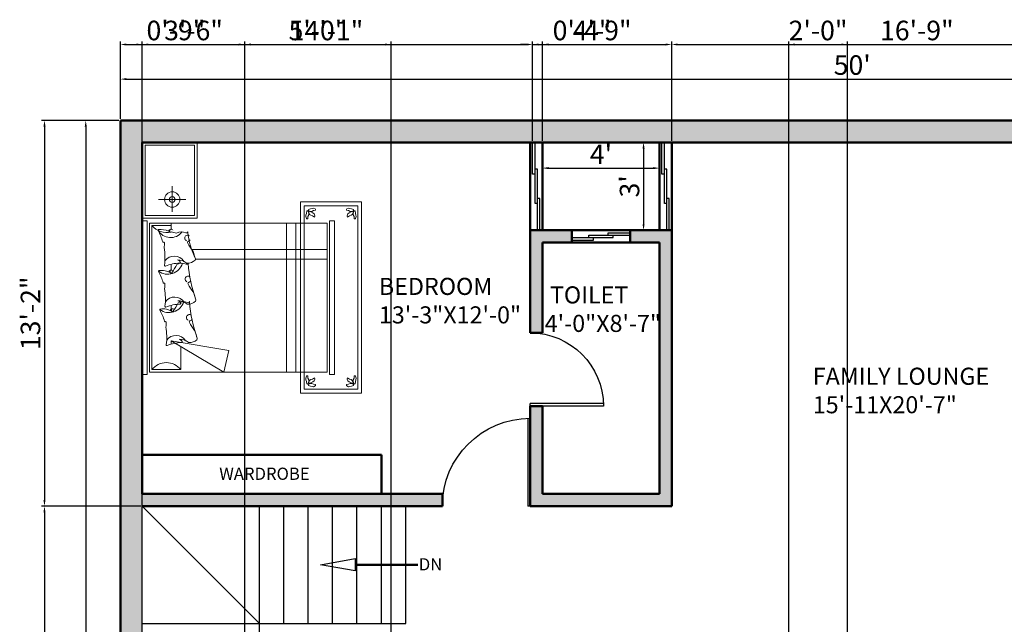
# Model space of a CAD drawing. Units: inches. Extents: x 1770 to 3141, y 984 to 1614.
# Tile 11 of 12: x 2468 to 2871, y 1359 to 1606. Entities that reach past the tile are written whole.
import ezdxf

# ---------------------------------------------------------------- set-up
doc = ezdxf.new("R2010")
doc.units = ezdxf.units.IN
for name, color, linetype, lineweight in [('A-ANNO-DIMS', 2, 'Continuous', 18), ('A-ANNO-TEXT', 7, 'Continuous', 18), ('A-AREA-IDEN', 3, 'Continuous', 18), ('A-DOOR', 4, 'Continuous', 25), ('A-FLOR-STRS', 7, 'Continuous', 25), ('A-FURN', 8, 'Continuous', 18), ('A-GLAZ', 5, 'Continuous', 25), ('A-WALL', 7, 'Continuous', 50), ('A-WALL-PATT', 8, 'Continuous', 13)]:
    doc.layers.add(name, color=color, linetype=linetype, lineweight=lineweight)
doc.styles.get("Standard").update_dxf_attribs({"font": 'arial.ttf'})
doc.dimstyles.new('ISO-25', dxfattribs={"dimtxt": 8, "dimasz": 2.5, "dimexe": 1.25, "dimexo": 0.625, "dimtad": 1, "dimdec": 1, "dimlunit": 3, "dimtxsty": 'Standard', "dimcen": 2.5, "dimclrt": 1, "dimadec": 0, "dimazin": 0, "dimtfac": 1, "dimtdec": 1, "dimtmove": 0, "dimatfit": 3, "dimfxl": 1, "dimarcsym": 0})

# ---------------------------------------------------------------- blocks, each defined once
blk = doc.blocks.new("D1 3'")
for p, q in [((0, 36), (0, 0)), ((1, 36), (1, 0)), ((0, 0), (1, 0))]:
    blk.add_line(p, q)
blk.add_arc((0, 0), 36, 0, 90)
blk = doc.blocks.new("D2 2'6")
for p, q in [((0, 30), (0, 0)), ((1, 30), (1, 0)), ((0, 0), (1, 0))]:
    blk.add_line(p, q)
blk.add_arc((0, 0), 30, 0, 90)
blk = doc.blocks.new('*D20')
at = {"layer": 'A-ANNO-DIMS', "color": 0, "lineweight": -2, "transparency": 16777216}
for p, q in [((2509.08, 1565.8), (2509.08, 1583.37)), ((3109.08, 1565.8), (3109.08, 1583.37)), ((2511.58, 1582.12), (3106.58, 1582.12))]:
    blk.add_line(p, q, dxfattribs=at)
at = {"layer": 'A-ANNO-DIMS', "color": 0, "transparency": 16777216}
for points in [[(2511.58, 1582.54), (2511.58, 1581.7), (2509.08, 1582.12)], [(3106.58, 1582.54), (3106.58, 1581.7), (3109.08, 1582.12)]]:
    blk.add_solid(points, dxfattribs=at)
at = {"layer": 'Defpoints', "color": 0, "transparency": 16777216}
for p in [(3109.08, 1582.12), (2509.08, 1565.18), (3109.08, 1565.18)]:
    blk.add_point(p, dxfattribs=at)
at = {"layer": 'A-ANNO-DIMS', "color": 0, "transparency": 16777216, "insert": (2809.08, 1586.83), "char_height": 8, "attachment_point": 5}
blk.add_mtext("50'", dxfattribs=at)
blk = doc.blocks.new('*D19')
at = {"layer": 'A-ANNO-DIMS', "color": 0, "lineweight": -2, "transparency": 16777216}
for p, q in [((2508.45, 1565.18), (2493.64, 1565.18)), ((2494.89, 1562.68), (2494.89, 1087.68)), ((2508.45, 1085.18), (2493.64, 1085.18))]:
    blk.add_line(p, q, dxfattribs=at)
at = {"layer": 'A-ANNO-DIMS', "color": 0, "transparency": 16777216}
for points in [[(2494.47, 1562.68), (2495.3, 1562.68), (2494.89, 1565.18)], [(2494.47, 1087.68), (2495.3, 1087.68), (2494.89, 1085.18)]]:
    blk.add_solid(points, dxfattribs=at)
at = {"layer": 'Defpoints', "color": 0, "transparency": 16777216}
for p in [(2509.08, 1565.18), (2494.89, 1085.18), (2509.08, 1085.18)]:
    blk.add_point(p, dxfattribs=at)
at = {"layer": 'A-ANNO-DIMS', "color": 0, "transparency": 16777216, "insert": (2490.18, 1325.18), "char_height": 8, "attachment_point": 5, "rotation": 90}
blk.add_mtext("40'", dxfattribs=at)
blk = doc.blocks.new('carpet-7')
at = {"color": 0, "linetype": 'ByBlock'}
for p, q in [((-1.0224, 0), (0, 0)), ((0, 0), (0, -0.54)), ((-1.694, -0.54), (-1.694, 0)), ((-1.694, 0), (-1.0224, 0)), ((-1.658, -0.5076), (-1.658, -0.0324)), ((-1.658, -0.0324), (-0.036, -0.0324)), ((-1.6304, -0.0896), (-1.6256, -0.0702)), ((-1.6256, -0.0702), (-1.6172, -0.0691)), ((-1.6172, -0.0691), (-1.6124, -0.0724)), ((-1.6112, -0.0562), (-1.6124, -0.0637)), ((-1.6124, -0.0637), (-1.6088, -0.068)), ((-1.6124, -0.0724), (-1.6064, -0.0886)), ((-1.5896, -0.0518), (-1.6112, -0.0562)), ((-1.6088, -0.068), (-1.5908, -0.0734)), ((-1.6088, -0.0788), (-1.6028, -0.0724)), ((-1.5992, -0.0961), (-1.6088, -0.0788)), ((-1.6028, -0.0724), (-1.5968, -0.0724)), ((-1.5968, -0.0724), (-1.5812, -0.081)), ((-1.5908, -0.0734), (-1.5764, -0.0724)), ((-1.5752, -0.0486), (-1.5896, -0.0518)), ((-1.5812, -0.081), (-1.5728, -0.0918)), ((-1.5764, -0.0724), (-1.5608, -0.0659)), ((-1.5608, -0.0464), (-1.5752, -0.0486)), ((-1.544, -0.0529), (-1.5608, -0.0464)), ((-1.5608, -0.0659), (-1.5404, -0.0637)), ((-1.5404, -0.0562), (-1.544, -0.0529)), ((-1.5404, -0.0637), (-1.5404, -0.0562)), ((-0.1512, -0.0562), (-0.1476, -0.0529)), ((-0.1512, -0.0637), (-0.1512, -0.0562)), ((-0.1308, -0.0659), (-0.1512, -0.0637)), ((-0.1476, -0.0529), (-0.1308, -0.0464)), ((-0.1308, -0.0464), (-0.1164, -0.0486)), ((-0.1152, -0.0724), (-0.1308, -0.0659)), ((-0.1104, -0.081), (-0.1188, -0.0918)), ((-0.1164, -0.0486), (-0.102, -0.0518)), ((-0.1008, -0.0734), (-0.1152, -0.0724)), ((-0.0948, -0.0724), (-0.1104, -0.081)), ((-0.102, -0.0518), (-0.0804, -0.0562)), ((-0.0828, -0.068), (-0.1008, -0.0734)), ((-0.0888, -0.0724), (-0.0948, -0.0724)), ((-0.0924, -0.0961), (-0.0828, -0.0788)), ((-0.0828, -0.0788), (-0.0888, -0.0724)), ((-0.0792, -0.0724), (-0.0852, -0.0886)), ((-0.0792, -0.0637), (-0.0828, -0.068)), ((-0.0804, -0.0562), (-0.0792, -0.0637)), ((-0.0744, -0.0691), (-0.0792, -0.0724)), ((-0.066, -0.0702), (-0.0744, -0.0691)), ((-0.0612, -0.0896), (-0.066, -0.0702)), ((-0.036, -0.0324), (-0.036, -0.5076)), ((-1.6364, -0.1156), (-1.634, -0.1026)), ((-1.6292, -0.1307), (-1.6364, -0.1156)), ((-1.634, -0.1026), (-1.6304, -0.0896)), ((-1.6256, -0.1339), (-1.6292, -0.1307)), ((-1.6172, -0.1339), (-1.6256, -0.1339)), ((-1.6148, -0.1156), (-1.6172, -0.1339)), ((-1.6076, -0.1015), (-1.6148, -0.1156)), ((-1.6064, -0.0886), (-1.6076, -0.1015)), ((-1.5932, -0.108), (-1.5992, -0.0961)), ((-1.5848, -0.1199), (-1.5932, -0.108)), ((-1.5692, -0.1274), (-1.5848, -0.1199)), ((-1.5728, -0.0918), (-1.568, -0.1069)), ((-1.5632, -0.1274), (-1.5692, -0.1274)), ((-1.568, -0.1069), (-1.5572, -0.1231)), ((-1.5572, -0.1231), (-1.5632, -0.1274)), ((-0.1236, -0.1069), (-0.1344, -0.1231)), ((-0.1344, -0.1231), (-0.1284, -0.1274)), ((-0.1284, -0.1274), (-0.1224, -0.1274)), ((-0.1188, -0.0918), (-0.1236, -0.1069)), ((-0.1224, -0.1274), (-0.1068, -0.1199)), ((-0.1068, -0.1199), (-0.0984, -0.108)), ((-0.0984, -0.108), (-0.0924, -0.0961)), ((-0.0852, -0.0886), (-0.084, -0.1015)), ((-0.084, -0.1015), (-0.0768, -0.1156)), ((-0.0768, -0.1156), (-0.0744, -0.1339)), ((-0.0744, -0.1339), (-0.066, -0.1339)), ((-0.066, -0.1339), (-0.0624, -0.1307)), ((-0.0624, -0.1307), (-0.0552, -0.1156)), ((-0.0576, -0.1026), (-0.0612, -0.0896)), ((-0.0552, -0.1156), (-0.0576, -0.1026)), ((-1.6292, -0.4093), (-1.6364, -0.4244)), ((-1.6364, -0.4244), (-1.634, -0.4374)), ((-1.6256, -0.4061), (-1.6292, -0.4093)), ((-1.6172, -0.4061), (-1.6256, -0.4061)), ((-1.6148, -0.4244), (-1.6172, -0.4061)), ((-1.6076, -0.4385), (-1.6148, -0.4244)), ((-1.5932, -0.432), (-1.5992, -0.4439)), ((-1.5848, -0.4201), (-1.5932, -0.432)), ((-1.5692, -0.4126), (-1.5848, -0.4201)), ((-1.5728, -0.4482), (-1.568, -0.4331)), ((-1.5632, -0.4126), (-1.5692, -0.4126)), ((-1.568, -0.4331), (-1.5572, -0.4169)), ((-1.5572, -0.4169), (-1.5632, -0.4126)), ((-0.1344, -0.4169), (-0.1284, -0.4126)), ((-0.1236, -0.4331), (-0.1344, -0.4169)), ((-0.1284, -0.4126), (-0.1224, -0.4126)), ((-0.1188, -0.4482), (-0.1236, -0.4331)), ((-0.1224, -0.4126), (-0.1068, -0.4201)), ((-0.1068, -0.4201), (-0.0984, -0.432)), ((-0.0984, -0.432), (-0.0924, -0.4439)), ((-0.084, -0.4385), (-0.0768, -0.4244)), ((-0.0768, -0.4244), (-0.0744, -0.4061)), ((-0.0744, -0.4061), (-0.066, -0.4061)), ((-0.066, -0.4061), (-0.0624, -0.4093)), ((-0.0624, -0.4093), (-0.0552, -0.4244)), ((-0.0552, -0.4244), (-0.0576, -0.4374)), ((-1.658, -0.5076), (-0.036, -0.5076)), ((-1.634, -0.4374), (-1.6304, -0.4504)), ((-1.6304, -0.4504), (-1.6256, -0.4698)), ((-1.6256, -0.4698), (-1.6172, -0.4709)), ((-1.6172, -0.4709), (-1.6124, -0.4676)), ((-1.6124, -0.4676), (-1.6064, -0.4514)), ((-1.6124, -0.4763), (-1.6088, -0.472)), ((-1.6112, -0.4838), (-1.6124, -0.4763)), ((-1.5896, -0.4882), (-1.6112, -0.4838)), ((-1.5992, -0.4439), (-1.6088, -0.4612)), ((-1.6088, -0.4612), (-1.6028, -0.4676)), ((-1.6088, -0.472), (-1.5908, -0.4666)), ((-1.6064, -0.4514), (-1.6076, -0.4385)), ((-1.6028, -0.4676), (-1.5968, -0.4676)), ((-1.5968, -0.4676), (-1.5812, -0.459)), ((-1.5908, -0.4666), (-1.5764, -0.4676)), ((-1.5752, -0.4914), (-1.5896, -0.4882)), ((-1.5812, -0.459), (-1.5728, -0.4482)), ((-1.5764, -0.4676), (-1.5608, -0.4741)), ((-1.5608, -0.4936), (-1.5752, -0.4914)), ((-1.5608, -0.4741), (-1.5404, -0.4763)), ((-1.544, -0.4871), (-1.5608, -0.4936)), ((-1.5404, -0.4838), (-1.544, -0.4871)), ((-1.5404, -0.4763), (-1.5404, -0.4838)), ((-0.1308, -0.4741), (-0.1512, -0.4763)), ((-0.1512, -0.4763), (-0.1512, -0.4838)), ((-0.1512, -0.4838), (-0.1476, -0.4871)), ((-0.1476, -0.4871), (-0.1308, -0.4936)), ((-0.1152, -0.4676), (-0.1308, -0.4741)), ((-0.1308, -0.4936), (-0.1164, -0.4914)), ((-0.1104, -0.459), (-0.1188, -0.4482)), ((-0.1164, -0.4914), (-0.102, -0.4882)), ((-0.1008, -0.4666), (-0.1152, -0.4676)), ((-0.0948, -0.4676), (-0.1104, -0.459)), ((-0.102, -0.4882), (-0.0804, -0.4838)), ((-0.0828, -0.472), (-0.1008, -0.4666)), ((-0.0888, -0.4676), (-0.0948, -0.4676)), ((-0.0924, -0.4439), (-0.0828, -0.4612)), ((-0.0828, -0.4612), (-0.0888, -0.4676)), ((-0.0852, -0.4514), (-0.084, -0.4385)), ((-0.0792, -0.4676), (-0.0852, -0.4514)), ((-0.0792, -0.4763), (-0.0828, -0.472)), ((-0.0804, -0.4838), (-0.0792, -0.4763)), ((-0.0744, -0.4709), (-0.0792, -0.4676)), ((-0.066, -0.4698), (-0.0744, -0.4709)), ((-0.0612, -0.4504), (-0.066, -0.4698)), ((-0.0576, -0.4374), (-0.0612, -0.4504)), ((0, -0.54), (-1.694, -0.54))]:
    blk.add_line(p, q, dxfattribs=at)
blk = doc.blocks.new('*D54')
at = {"layer": 'A-ANNO-DIMS', "color": 0, "lineweight": -2, "transparency": 16777216}
for p, q in [((2682.08, 1547.77), (2682.08, 1544.4)), ((2730.08, 1547.77), (2730.08, 1544.4)), ((2684.58, 1545.65), (2727.58, 1545.65))]:
    blk.add_line(p, q, dxfattribs=at)
at = {"layer": 'A-ANNO-DIMS', "color": 0, "transparency": 16777216}
for points in [[(2684.58, 1546.07), (2684.58, 1545.23), (2682.08, 1545.65)], [(2727.58, 1546.07), (2727.58, 1545.23), (2730.08, 1545.65)]]:
    blk.add_solid(points, dxfattribs=at)
at = {"layer": 'Defpoints', "color": 0, "transparency": 16777216}
for p in [(2682.08, 1548.4), (2730.08, 1548.4), (2730.08, 1545.65)]:
    blk.add_point(p, dxfattribs=at)
at = {"layer": 'A-ANNO-DIMS', "color": 0, "transparency": 16777216, "insert": (2706.08, 1550.28), "char_height": 8, "attachment_point": 5}
blk.add_mtext("4'", dxfattribs=at)
blk = doc.blocks.new('*D55')
at = {"layer": 'A-ANNO-DIMS', "color": 0, "lineweight": -2, "transparency": 16777216}
for p, q in [((2722.45, 1556.18), (2724.79, 1556.18)), ((2723.54, 1553.68), (2723.54, 1522.68)), ((2722.45, 1520.18), (2724.79, 1520.18))]:
    blk.add_line(p, q, dxfattribs=at)
at = {"layer": 'A-ANNO-DIMS', "color": 0, "transparency": 16777216}
for points in [[(2723.12, 1553.68), (2723.96, 1553.68), (2723.54, 1556.18)], [(2723.12, 1522.68), (2723.96, 1522.68), (2723.54, 1520.18)]]:
    blk.add_solid(points, dxfattribs=at)
at = {"layer": 'Defpoints', "color": 0, "transparency": 16777216}
for p in [(2721.82, 1556.18), (2721.82, 1520.18), (2723.54, 1520.18)]:
    blk.add_point(p, dxfattribs=at)
at = {"layer": 'A-ANNO-DIMS', "color": 0, "transparency": 16777216, "insert": (2718.83, 1538.18), "char_height": 8, "attachment_point": 5, "rotation": 90}
blk.add_mtext("3'", dxfattribs=at)
blk = doc.blocks.new('BED-DOUBLE')
for p, q in [((3.94, 1.97), (3.94, 61.02)), ((3.94, 61.02), (11.81, 61.02)), ((11.81, 62.01), (11.81, 59.48)), ((59.06, 0.98), (59.06, 62.01)), ((62.99, 0.98), (62.99, 62.01)), ((20.58, 51.18), (75.79, 51.18)), ((11.81, 45.13), (11.81, 42.7)), ((21.83, 47.24), (75.79, 47.24)), ((11.81, 28.3), (11.81, 26.75)), ((11.81, 13.78), (33.46, 0.98)), ((35.43, 9.84), (11.81, 13.78)), ((11.81, 12.41), (11.81, 13.78)), ((15.75, 1.97), (15.75, 11.45)), ((33.46, 0.98), (35.43, 9.84)), ((3.94, 1.97), (15.75, 1.97))]:
    blk.add_line(p, q)
for points in [[(1.97, 0), (1.97, 62.99), (0, 62.99), (0, 0)], [(75.79, 62.01), (2.95, 62.01), (2.95, 0.98), (75.79, 0.98)], [(78.74, 0), (78.74, 62.99), (76.77, 62.99), (76.77, 0)]]:
    blk.add_lwpolyline(points, close=True)
for centre, radius, start, end in [((9.84, 65.6), 7.47, 217.7826, 285.2747), ((6.72, 59.06), 0.283, 97.124, 208.2114), ((6.72, 59.06), 0.283, 97.124, 208.2114), ((11.6, 61.98), 5.92, 209.3598, 322.4281), ((-14.44, 47.71), 23.73, 16.2196, 28.2114), ((7.62, 51.84), 7.55, 66.1093, 97.124), ((11.74, 58.34), 1.13, 52.662, 159.1573), ((74.55, 55.49), 63.42, 176.4982, 177.2888), ((11.63, 58.56), 0.283, 218.8315, 325.8329), ((16.48, 74.25), 16.51, 253.7524, 261.4605), ((-45.71, 34.29), 63.42, 22.7018, 22.7206), ((16.03, 53.78), 4.59, 67.1663, 115.7613), ((18.58, 55.86), 1.2, 52.3565, 245.7762), ((18.03, 58.54), 0.567, 247.1663, 4.3422), ((51.64, 61.93), 33.22, 186.224, 206.0326), ((8.62, 54.41), 0.283, 196.2196, 290.689), ((8.82, 53.88), 0.283, 359.3085, 110.689), ((-2.22, 54.02), 11.32, 349.4168, 359.3085), ((19.09, 54.05), 0.567, 102.6426, 209.049), ((41.54, 66.52), 26.25, 209.049, 217.3823), ((18.84, 55.16), 0.567, 282.6426, 292.7015), ((18.58, 55.79), 1.26, 292.7015, 327.1556), ((-14.44, 47.71), 23.73, 352.7248, 10.2702), ((13.07, 43.78), 4.71, 32.7628, 143.8922), ((20.28, 50.19), 0.567, 16.386, 43.7955), ((77.39, 66.98), 58.96, 196.386, 199.4465), ((10.39, 47.46), 6.39, 233.8947, 342.3952), ((9.38, 44.67), 0.283, 172.7248, 290.959), ((16.23, 26.77), 18.88, 92.7363, 110.959), ((-34.15, 72.98), 55.83, 325.8329, 330.0245), ((16.21, 40.94), 4.59, 67.1663, 115.7613), ((14.36, 41.08), 5.89, 51.6071, 89.7845), ((13.92, 45.16), 1.87, 28.2985, 75.7891), ((15.32, 45.91), 0.283, 272.7363, 28.2985), ((18.22, 45.7), 0.567, 247.1663, 4.3422), ((18.37, 46.14), 0.567, 231.6071, 267.3377), ((18.56, 50.2), 4.62, 267.3377, 311.666), ((77.57, 50.21), 58.96, 184.5852, 199.4465), ((21.25, 47.17), 0.567, 311.666, 19.4465), ((6.91, 42.28), 0.283, 97.124, 208.2114), ((6.91, 42.28), 0.283, 97.124, 208.2114), ((-14.25, 30.93), 23.73, 16.2196, 28.2114), ((7.81, 35.07), 7.55, 59.9211, 97.124), ((11.93, 41.57), 1.13, 52.662, 159.1573), ((74.73, 38.72), 63.42, 176.4982, 177.2888), ((11.81, 41.78), 0.283, 218.8315, 325.8329), ((-45.53, 17.51), 63.42, 22.7018, 22.7206), ((8.8, 37.64), 0.283, 196.2196, 290.689), ((9, 37.11), 0.283, 359.3085, 110.689), ((-2.03, 37.24), 11.32, 349.4168, 359.3085), ((18.76, 39.09), 1.2, 52.3565, 245.7762), ((19.28, 37.27), 0.567, 102.6426, 209.049), ((41.73, 49.74), 26.25, 209.049, 217.3823), ((19.03, 38.38), 0.567, 282.6426, 292.7015), ((18.76, 39.02), 1.26, 292.7015, 327.1556), ((-14.25, 30.93), 23.73, 352.7248, 10.2702), ((20.46, 33.41), 0.567, 16.386, 43.7955), ((77.57, 50.21), 58.96, 196.386, 199.4465), ((10.93, 31.72), 6.39, 233.8947, 342.3952), ((13.25, 27), 4.71, 32.7628, 143.8922), ((16.42, 9.99), 18.88, 92.7363, 110.959), ((-33.61, 57.23), 55.83, 325.8329, 330.0245), ((14.54, 24.31), 5.89, 51.6071, 89.7845), ((14.11, 28.38), 1.87, 28.2985, 75.7891), ((16.75, 25.2), 4.59, 67.1663, 115.7613), ((15.5, 29.14), 0.283, 272.7363, 28.2985), ((18.56, 29.37), 0.567, 231.6071, 267.3377), ((18.75, 29.96), 0.567, 247.1663, 4.3422), ((18.74, 33.42), 4.62, 267.3377, 311.666), ((78.11, 34.46), 58.96, 184.5852, 199.4465), ((21.44, 30.39), 0.567, 311.666, 19.4465), ((7.44, 26.53), 0.283, 97.124, 208.2114), ((7.44, 26.53), 0.283, 97.124, 208.2114), ((-13.71, 15.19), 23.73, 16.2196, 28.2114), ((8.35, 19.32), 7.55, 59.9211, 97.124), ((9.56, 27.89), 0.283, 172.7248, 290.959), ((12.47, 25.82), 1.13, 52.662, 159.1573), ((75.27, 22.97), 63.42, 176.4982, 177.2888), ((12.35, 26.04), 0.283, 218.8315, 325.8329), ((-44.99, 1.77), 63.42, 22.7018, 22.7206), ((19.3, 23.34), 1.2, 52.3565, 245.7762), ((9.34, 21.89), 0.283, 196.2196, 290.689), ((9.54, 21.36), 0.283, 359.3085, 110.689), ((-1.49, 21.49), 11.32, 349.4168, 359.3085), ((19.82, 21.53), 0.567, 102.6426, 209.049), ((42.27, 34), 26.25, 209.049, 217.3823), ((19.57, 22.63), 0.567, 282.6426, 292.7015), ((19.3, 23.27), 1.26, 292.7015, 327.1556), ((-13.71, 15.19), 23.73, 352.7248, 10.2702), ((21, 17.67), 0.567, 16.386, 43.7955), ((78.11, 34.46), 58.96, 196.386, 199.4465), ((10.1, 12.14), 0.283, 172.7248, 290.959), ((13.79, 11.26), 4.71, 32.7628, 143.8922), ((16.96, -5.75), 18.88, 92.7363, 110.959), ((15.08, 8.56), 5.89, 51.6071, 89.7845), ((14.65, 12.64), 1.87, 28.2985, 75.7891), ((16.04, 13.39), 0.283, 272.7363, 28.2985), ((19.09, 13.62), 0.567, 231.6071, 267.3377), ((19.28, 17.67), 4.62, 267.3377, 311.666), ((21.98, 14.64), 0.567, 311.666, 19.4465), ((9.84, -2.61), 7.47, 37.7826, 142.2174)]:
    blk.add_arc(centre, radius, start, end)
blk = doc.blocks.new('*D122')
at = {"layer": 'A-ANNO-DIMS', "color": 0, "lineweight": -2, "transparency": 16777216}
for p, q in [((2509.08, 1565.8), (2509.08, 1597.53)), ((2511.58, 1596.28), (2675.58, 1596.28)), ((2678.08, 1556.8), (2678.08, 1597.53))]:
    blk.add_line(p, q, dxfattribs=at)
at = {"layer": 'A-ANNO-DIMS', "color": 0, "transparency": 16777216}
for points in [[(2511.58, 1596.7), (2511.58, 1595.86), (2509.08, 1596.28)], [(2675.58, 1596.7), (2675.58, 1595.86), (2678.08, 1596.28)]]:
    blk.add_solid(points, dxfattribs=at)
at = {"layer": 'Defpoints', "color": 0, "transparency": 16777216}
for p in [(2678.08, 1596.28), (2509.08, 1565.18), (2678.08, 1556.18)]:
    blk.add_point(p, dxfattribs=at)
at = {"layer": 'A-ANNO-DIMS', "color": 1, "transparency": 16777216, "insert": (2593.58, 1600.92), "char_height": 8, "attachment_point": 5}
blk.add_mtext('14\'-1"', dxfattribs=at)
blk = doc.blocks.new('*D123')
at = {"layer": 'A-ANNO-DIMS', "color": 0, "lineweight": -2, "transparency": 16777216}
for p, q in [((2678.08, 1556.8), (2678.08, 1597.53)), ((2680.58, 1596.28), (2732.58, 1596.28)), ((2735.08, 1556.8), (2735.08, 1597.53))]:
    blk.add_line(p, q, dxfattribs=at)
at = {"layer": 'A-ANNO-DIMS', "color": 0, "transparency": 16777216}
for points in [[(2680.58, 1596.7), (2680.58, 1595.86), (2678.08, 1596.28)], [(2732.58, 1596.7), (2732.58, 1595.86), (2735.08, 1596.28)]]:
    blk.add_solid(points, dxfattribs=at)
at = {"layer": 'Defpoints', "color": 0, "transparency": 16777216}
for p in [(2735.08, 1596.28), (2678.08, 1556.18), (2735.08, 1556.18)]:
    blk.add_point(p, dxfattribs=at)
at = {"layer": 'A-ANNO-DIMS', "color": 1, "transparency": 16777216, "insert": (2706.58, 1600.99), "char_height": 8, "attachment_point": 5}
blk.add_mtext('4\'-9"', dxfattribs=at)
blk = doc.blocks.new('*D124')
at = {"layer": 'A-ANNO-DIMS', "color": 0, "lineweight": -2, "transparency": 16777216}
for p, q in [((2735.08, 1556.8), (2735.08, 1597.53)), ((2737.58, 1596.28), (2933.58, 1596.28)), ((2936.08, 1565.8), (2936.08, 1597.53))]:
    blk.add_line(p, q, dxfattribs=at)
at = {"layer": 'A-ANNO-DIMS', "color": 0, "transparency": 16777216}
for points in [[(2737.58, 1596.7), (2737.58, 1595.86), (2735.08, 1596.28)], [(2933.58, 1596.7), (2933.58, 1595.86), (2936.08, 1596.28)]]:
    blk.add_solid(points, dxfattribs=at)
at = {"layer": 'Defpoints', "color": 0, "transparency": 16777216}
for p in [(2936.08, 1596.28), (2936.08, 1565.18), (2735.08, 1556.18)]:
    blk.add_point(p, dxfattribs=at)
at = {"layer": 'A-ANNO-DIMS', "color": 1, "transparency": 16777216, "insert": (2835.58, 1600.99), "char_height": 8, "attachment_point": 5}
blk.add_mtext('16\'-9"', dxfattribs=at)
blk = doc.blocks.new('*D126')
at = {"layer": 'A-ANNO-DIMS', "color": 0, "lineweight": -2, "transparency": 16777216}
for p, q in [((2509.08, 1565.8), (2509.08, 1597.53)), ((2511.58, 1596.28), (2515.58, 1596.28)), ((2518.08, 1556.8), (2518.08, 1597.53)), ((2518.08, 1596.28), (2543.09, 1596.28))]:
    blk.add_line(p, q, dxfattribs=at)
at = {"layer": 'A-ANNO-DIMS', "color": 0, "transparency": 16777216}
for points in [[(2511.58, 1596.7), (2511.58, 1595.86), (2509.08, 1596.28)], [(2515.58, 1596.7), (2515.58, 1595.86), (2518.08, 1596.28)]]:
    blk.add_solid(points, dxfattribs=at)
at = {"layer": 'Defpoints', "color": 0, "transparency": 16777216}
for p in [(2518.08, 1596.28), (2509.08, 1565.18), (2518.08, 1556.18)]:
    blk.add_point(p, dxfattribs=at)
at = {"layer": 'A-ANNO-DIMS', "color": 1, "transparency": 16777216, "insert": (2531.84, 1600.99), "char_height": 8, "attachment_point": 5}
blk.add_mtext('0\'-9"', dxfattribs=at)
blk = doc.blocks.new('*D127')
at = {"layer": 'A-ANNO-DIMS', "color": 0, "lineweight": -2, "transparency": 16777216}
for p, q in [((2675.58, 1596.28), (2673.08, 1596.28)), ((2678.08, 1556.8), (2678.08, 1597.53)), ((2678.08, 1596.28), (2682.08, 1596.28)), ((2682.08, 1556.8), (2682.08, 1597.53)), ((2684.58, 1596.28), (2709.59, 1596.28))]:
    blk.add_line(p, q, dxfattribs=at)
at = {"layer": 'A-ANNO-DIMS', "color": 0, "transparency": 16777216}
for points in [[(2675.58, 1596.7), (2675.58, 1595.86), (2678.08, 1596.28)], [(2684.58, 1596.7), (2684.58, 1595.86), (2682.08, 1596.28)]]:
    blk.add_solid(points, dxfattribs=at)
at = {"layer": 'Defpoints', "color": 0, "transparency": 16777216}
for p in [(2682.08, 1596.28), (2678.08, 1556.18), (2682.08, 1556.18)]:
    blk.add_point(p, dxfattribs=at)
at = {"layer": 'A-ANNO-DIMS', "color": 1, "transparency": 16777216, "insert": (2698.34, 1600.99), "char_height": 8, "attachment_point": 5}
blk.add_mtext('0\'-4"', dxfattribs=at)
blk = doc.blocks.new('*D128')
at = {"layer": 'A-ANNO-DIMS', "color": 0, "lineweight": -2, "transparency": 16777216}
for p, q in [((2508.45, 1565.18), (2476.73, 1565.18)), ((2477.98, 1562.68), (2477.98, 1409.68)), ((2517.45, 1407.18), (2476.73, 1407.18))]:
    blk.add_line(p, q, dxfattribs=at)
at = {"layer": 'A-ANNO-DIMS', "color": 0, "transparency": 16777216}
for points in [[(2477.56, 1562.68), (2478.4, 1562.68), (2477.98, 1565.18)], [(2477.56, 1409.68), (2478.4, 1409.68), (2477.98, 1407.18)]]:
    blk.add_solid(points, dxfattribs=at)
at = {"layer": 'Defpoints', "color": 0, "transparency": 16777216}
for p in [(2509.08, 1565.18), (2477.98, 1407.18), (2518.08, 1407.18)]:
    blk.add_point(p, dxfattribs=at)
at = {"layer": 'A-ANNO-DIMS', "color": 1, "transparency": 16777216, "insert": (2473.27, 1486.18), "char_height": 8, "attachment_point": 5, "rotation": 90}
blk.add_mtext('13\'-2"', dxfattribs=at)
blk = doc.blocks.new('*D129')
at = {"layer": 'A-ANNO-DIMS', "color": 0, "lineweight": -2, "transparency": 16777216}
for p, q in [((2517.45, 1407.18), (2476.73, 1407.18)), ((2477.98, 1404.68), (2477.98, 1248.68)), ((2517.45, 1246.18), (2476.73, 1246.18))]:
    blk.add_line(p, q, dxfattribs=at)
at = {"layer": 'A-ANNO-DIMS', "color": 0, "transparency": 16777216}
for points in [[(2477.56, 1404.68), (2478.4, 1404.68), (2477.98, 1407.18)], [(2477.56, 1248.68), (2478.4, 1248.68), (2477.98, 1246.18)]]:
    blk.add_solid(points, dxfattribs=at)
at = {"layer": 'Defpoints', "color": 0, "transparency": 16777216}
for p in [(2518.08, 1407.18), (2477.98, 1246.18), (2518.08, 1246.18)]:
    blk.add_point(p, dxfattribs=at)
at = {"layer": 'A-ANNO-DIMS', "color": 1, "transparency": 16777216, "insert": (2473.27, 1326.68), "char_height": 8, "attachment_point": 5, "rotation": 90}
blk.add_mtext('13\'-5"', dxfattribs=at)
blk = doc.blocks.new('*D135')
at = {"layer": 'A-ANNO-DIMS', "color": 0, "lineweight": -2, "transparency": 16777216}
for p, q in [((2518.08, 1094.8), (2518.08, 1597.53)), ((2520.58, 1596.28), (2557.58, 1596.28)), ((2560.08, 1094.8), (2560.08, 1597.53))]:
    blk.add_line(p, q, dxfattribs=at)
at = {"layer": 'A-ANNO-DIMS', "color": 0, "transparency": 16777216}
for points in [[(2520.58, 1596.7), (2520.58, 1595.86), (2518.08, 1596.28)], [(2557.58, 1596.7), (2557.58, 1595.86), (2560.08, 1596.28)]]:
    blk.add_solid(points, dxfattribs=at)
at = {"layer": 'Defpoints', "color": 0, "transparency": 16777216}
for p in [(2560.08, 1596.28), (2518.08, 1094.18), (2560.08, 1094.18)]:
    blk.add_point(p, dxfattribs=at)
at = {"layer": 'A-ANNO-DIMS', "color": 1, "transparency": 16777216, "insert": (2539.08, 1600.99), "char_height": 8, "attachment_point": 5}
blk.add_mtext('3\'-6"', dxfattribs=at)
blk = doc.blocks.new('*D136')
at = {"layer": 'A-ANNO-DIMS', "color": 0, "lineweight": -2, "transparency": 16777216}
for p, q in [((2560.08, 1094.8), (2560.08, 1597.53)), ((2562.58, 1596.28), (2617.58, 1596.28)), ((2620.08, 1094.8), (2620.08, 1597.53))]:
    blk.add_line(p, q, dxfattribs=at)
at = {"layer": 'A-ANNO-DIMS', "color": 0, "transparency": 16777216}
for points in [[(2562.58, 1596.7), (2562.58, 1595.86), (2560.08, 1596.28)], [(2617.58, 1596.7), (2617.58, 1595.86), (2620.08, 1596.28)]]:
    blk.add_solid(points, dxfattribs=at)
at = {"layer": 'Defpoints', "color": 0, "transparency": 16777216}
for p in [(2620.08, 1596.28), (2560.08, 1094.18), (2620.08, 1094.18)]:
    blk.add_point(p, dxfattribs=at)
at = {"layer": 'A-ANNO-DIMS', "color": 1, "transparency": 16777216, "insert": (2590.08, 1600.99), "char_height": 8, "attachment_point": 5}
blk.add_mtext('5\'-0"', dxfattribs=at)
blk = doc.blocks.new('*D137')
at = {"layer": 'A-ANNO-DIMS', "color": 0, "lineweight": -2, "transparency": 16777216}
for p, q in [((2783.08, 1094.8), (2783.08, 1597.53)), ((2785.58, 1596.28), (2804.58, 1596.28)), ((2807.08, 1094.8), (2807.08, 1597.53))]:
    blk.add_line(p, q, dxfattribs=at)
at = {"layer": 'A-ANNO-DIMS', "color": 0, "transparency": 16777216}
for points in [[(2785.58, 1596.7), (2785.58, 1595.86), (2783.08, 1596.28)], [(2804.58, 1596.7), (2804.58, 1595.86), (2807.08, 1596.28)]]:
    blk.add_solid(points, dxfattribs=at)
at = {"layer": 'Defpoints', "color": 0, "transparency": 16777216}
for p in [(2807.08, 1596.28), (2783.08, 1094.18), (2807.08, 1094.18)]:
    blk.add_point(p, dxfattribs=at)
at = {"layer": 'A-ANNO-DIMS', "color": 1, "transparency": 16777216, "insert": (2795.08, 1600.99), "char_height": 8, "attachment_point": 5}
blk.add_mtext('2\'-0"', dxfattribs=at)

msp = doc.modelspace()

# ---------------------------------------------------------------- hatches: boundary and pattern name
at = {"layer": 'A-WALL-PATT'}
h = msp.add_hatch(color=256, dxfattribs=at)
h.dxf.hatch_style = 1
h.paths.add_polyline_path([(2936.08, 1565.18), (2509.08, 1565.18), (2509.08, 1100.18), (2518.08, 1100.18), (2518.08, 1125.25), (2518.08, 1246.18), (2662.08, 1246.18), (2662.08, 1251.18), (2518.08, 1251.18), (2518.08, 1407.18), (2641.08, 1407.18), (2641.08, 1412.18), (2518.08, 1412.18), (2518.08, 1556.18), (2540.6, 1556.18), (2931.08, 1556.18), (2931.08, 1520.18), (2936.08, 1520.18)])
h.paths.add_polyline_path([(2560.08, 1094.18), (2518.08, 1094.18), (2518.08, 1085.18), (2560.08, 1085.18)])
h.paths.add_polyline_path([(2662.08, 1094.18), (2620.08, 1094.18), (2620.08, 1085.18), (2662.08, 1085.18)])
h.paths.add_polyline_path([(2783.08, 1094.18), (2707.08, 1094.18), (2707.08, 1085.18), (2783.08, 1085.18)])
h.paths.add_polyline_path([(2703.08, 1179.18), (2698.08, 1179.18), (2698.08, 1100.18), (2703.08, 1100.18)], flags=16)
h.paths.add_polyline_path([(2813.08, 1094.18), (2807.08, 1094.18), (2807.08, 1085.18), (2813.08, 1085.18)])
h.paths.add_polyline_path([(2822.08, 1300.18), (2834.08, 1300.18), (2834.08, 1309.18), (2813.08, 1309.18), (2813.08, 1251.18), (2698.08, 1251.18), (2698.08, 1215.18), (2698.08, 1209.18), (2703.08, 1209.18), (2703.08, 1246.18), (2813.08, 1246.18), (2813.08, 1167.18), (2733.08, 1167.18), (2733.08, 1162.18), (2813.08, 1162.18), (2813.08, 1100.18), (2822.08, 1100.18)], flags=17)
h.paths.add_polyline_path([(2936.08, 1376.18), (2931.08, 1376.18), (2931.08, 1309.18), (2918.08, 1309.18), (2918.08, 1300.18), (2936.08, 1300.18)], flags=17)
h.paths.add_polyline_path([(2735.08, 1520.18), (2718.08, 1520.18), (2718.08, 1515.18), (2730.08, 1515.18), (2730.08, 1412.18), (2682.08, 1412.18), (2682.08, 1448.18), (2677.08, 1448.18), (2677.08, 1407.18), (2735.08, 1407.18)], flags=17)
h.paths.add_polyline_path([(2682.08, 1515.18), (2694.08, 1515.18), (2694.08, 1520.18), (2677.08, 1520.18), (2677.08, 1478.18), (2682.08, 1478.18)], flags=16)

# ---------------------------------------------------------------- linework, layer by layer
at = {"layer": 'A-FLOR-STRS'}
for p, q in [((2518.08, 1251.18), (2518.08, 1407.18)), ((2518.08, 1407.18), (2566.08, 1359.18)), ((2566.08, 1251.18), (2566.08, 1407.18)), ((2576.08, 1359.18), (2576.08, 1407.18)), ((2586.08, 1359.18), (2586.08, 1407.18)), ((2596.08, 1359.18), (2596.08, 1407.18)), ((2606.08, 1359.18), (2606.08, 1407.18)), ((2616.08, 1359.18), (2616.08, 1407.18)), ((2626.08, 1359.18), (2626.08, 1407.18)), ((2518.08, 1359.18), (2626.08, 1359.18))]:
    msp.add_line(p, q, dxfattribs=at)
msp.add_lwpolyline([(2591.17, 1383.18), (2605.32, 1385.73), (2605.32, 1380.63)], close=True, dxfattribs=at)
at = {"layer": 'A-FURN'}
for p, q in [((2530.34, 1538.32), (2530.34, 1527.72)), ((2524.71, 1532.79), (2535.93, 1532.79))]:
    msp.add_line(p, q, dxfattribs=at)
for points in [[(2540.6, 1525.1), (2518.08, 1525.1), (2518.08, 1556.18), (2540.6, 1556.18)], [(2539.42, 1526.28), (2519.26, 1526.28), (2519.26, 1555), (2539.42, 1555)]]:
    msp.add_lwpolyline(points, close=True, dxfattribs=at)
for radius in [3.15, 1.18]:
    msp.add_circle((2530.34, 1532.79), radius, dxfattribs=at)
at = {"layer": 'A-GLAZ'}
for p, q in [((2678.08, 1543.18), (2678.08, 1556.18)), ((2679.08, 1531.18), (2679.08, 1556.18)), ((2731.08, 1543.18), (2731.08, 1556.18)), ((2732.08, 1531.18), (2732.08, 1556.18)), ((2679.08, 1543.18), (2678.08, 1543.18)), ((2680.08, 1545.18), (2679.08, 1545.18)), ((2680.08, 1520.18), (2680.08, 1545.18)), ((2732.08, 1543.18), (2731.08, 1543.18)), ((2733.08, 1545.18), (2732.08, 1545.18)), ((2733.08, 1520.18), (2733.08, 1545.18)), ((2680.08, 1531.18), (2679.08, 1531.18)), ((2681.08, 1533.18), (2680.08, 1533.18)), ((2681.08, 1520.18), (2681.08, 1533.18)), ((2733.08, 1531.18), (2732.08, 1531.18)), ((2734.08, 1533.18), (2733.08, 1533.18)), ((2734.08, 1520.18), (2734.08, 1533.18)), ((2701.08, 1517.18), (2701.08, 1518.18)), ((2701.08, 1518.18), (2718.08, 1518.18)), ((2709.08, 1518.18), (2709.08, 1519.18)), ((2709.08, 1519.18), (2718.08, 1519.18)), ((2711.08, 1517.18), (2711.08, 1518.18)), ((2694.08, 1517.18), (2711.08, 1517.18)), ((2694.08, 1516.18), (2703.08, 1516.18)), ((2703.08, 1516.18), (2703.08, 1517.18))]:
    msp.add_line(p, q, dxfattribs=at)
at = {"layer": 'A-WALL'}
for p, q in [((2509.08, 1565.18), (3109.08, 1565.18)), ((2509.08, 1043.18), (2509.08, 1565.18)), ((2518.08, 1556.18), (2931.08, 1556.18)), ((2518.08, 1412.18), (2518.08, 1556.18)), ((2677.08, 1478.18), (2677.08, 1556.18)), ((2682.08, 1520.18), (2682.08, 1556.18)), ((2730.08, 1520.18), (2730.08, 1556.18)), ((2735.08, 1556.18), (2735.08, 1407.18)), ((2677.08, 1520.18), (2735.08, 1520.18)), ((2694.08, 1520.18), (2694.08, 1515.18)), ((2718.08, 1520.18), (2718.08, 1515.18)), ((2682.08, 1515.18), (2730.08, 1515.18)), ((2682.08, 1478.18), (2682.08, 1515.18)), ((2730.08, 1412.18), (2730.08, 1515.18)), ((2682.08, 1478.18), (2677.08, 1478.18)), ((2677.08, 1407.18), (2677.08, 1448.18)), ((2682.08, 1448.18), (2677.08, 1448.18)), ((2682.08, 1412.18), (2682.08, 1448.18)), ((2518.08, 1428.18), (2616.08, 1428.18)), ((2616.08, 1412.18), (2616.08, 1428.18)), ((2518.08, 1412.18), (2641.08, 1412.18)), ((2641.08, 1407.18), (2641.08, 1412.18)), ((2682.08, 1412.18), (2730.08, 1412.18)), ((2518.08, 1407.18), (2641.08, 1407.18)), ((2677.08, 1407.18), (2735.08, 1407.18)), ((2605.32, 1383.18), (2631.05, 1383.18))]:
    msp.add_line(p, q, dxfattribs=at)

# ---------------------------------------------------------------- block references
at = {"layer": 'A-DOOR', "xscale": -1, "rotation": 270}
msp.add_blockref("D2 2'6", (2677.08, 1448.18), dxfattribs=at)
at = {"layer": 'A-DOOR', "xscale": -1}
msp.add_blockref("D1 3'", (2677.08, 1407.18), dxfattribs=at)
at = {"layer": 'A-FURN', "xscale": 46.2750735389499, "yscale": 46.2750735389499, "zscale": 46.2750735389499, "rotation": 90}
msp.add_blockref('carpet-7', (2582.92, 1531.82), dxfattribs=at)
at = {"layer": 'A-FURN'}
msp.add_blockref('BED-DOUBLE', (2518.08, 1461.13), dxfattribs=at)

# ---------------------------------------------------------------- texts
at = {"layer": 'A-ANNO-TEXT', "insert": (2641.04, 1385.86), "char_height": 5, "attachment_point": 3}
msp.add_mtext_dynamic_manual_height_columns('{DN}', width=10.7355, gutter_width=12.5, heights=[0], dxfattribs=at)
at = {"layer": 'A-AREA-IDEN', "attachment_point": 1}
for s, insert, char_height in [('BEDROOM\\P13\'-3"X12\'-0"', (2615.06, 1500.7), 7), ('  TOILET\\P 4\'-0"X8\'-7"', (2680.89, 1497.22), 7), ('FAMILY LOUNGE\\P15\'-11X20\'-7"', (2792.92, 1463.9), 7), ('WARDROBE', (2549.61, 1422.96), 5)]:
    msp.add_mtext_dynamic_manual_height_columns(s, width=86.9528, gutter_width=12.5, heights=[0], dxfattribs=dict(at, insert=insert, char_height=char_height))

# ---------------------------------------------------------------- dimensions: what is measured, and where the dimension line sits
at = {"layer": 'A-ANNO-DIMS'}
for base, p1, p2, override, picture, middle in [((2518.08, 1596.28), (2509.08, 1565.18), (2518.08, 1556.18), {"dimdec": 1, "dimlfac": 1, "dimrnd": 0, "dimzin": 1, "dimdsep": 46, "dimlunit": 4, "dimfrac": 2}, '*D126', (2531.84, 1600.99)), ((2678.08, 1596.28), (2509.08, 1565.18), (2678.08, 1556.18), {"dimdec": 1, "dimlfac": 1, "dimrnd": 0, "dimzin": 1, "dimdsep": 46, "dimlunit": 4, "dimfrac": 2}, '*D122', (2593.58, 1600.92)), ((2560.08, 1596.28), (2518.08, 1094.18), (2560.08, 1094.18), {"dimdec": 1, "dimlfac": 1, "dimrnd": 0, "dimzin": 1, "dimdsep": 46, "dimlunit": 4, "dimfrac": 2}, '*D135', (2539.08, 1600.99)), ((2620.08, 1596.28), (2560.08, 1094.18), (2620.08, 1094.18), {"dimdec": 1, "dimlfac": 1, "dimrnd": 0, "dimzin": 1, "dimdsep": 46, "dimlunit": 4, "dimfrac": 2}, '*D136', (2590.08, 1600.99)), ((2682.08, 1596.28), (2678.08, 1556.18), (2682.08, 1556.18), {"dimdec": 1, "dimlfac": 1, "dimrnd": 0, "dimzin": 1, "dimdsep": 46, "dimlunit": 4, "dimfrac": 2}, '*D127', (2698.34, 1600.99)), ((2735.08, 1596.28), (2678.08, 1556.18), (2735.08, 1556.18), {"dimdec": 1, "dimlfac": 1, "dimrnd": 0, "dimzin": 1, "dimdsep": 46, "dimlunit": 4, "dimfrac": 2}, '*D123', (2706.58, 1600.99)), ((2936.08, 1596.28), (2735.08, 1556.18), (2936.08, 1565.18), {"dimdec": 1, "dimlfac": 1, "dimrnd": 0, "dimzin": 1, "dimdsep": 46, "dimlunit": 4, "dimfrac": 2}, '*D124', (2835.58, 1600.99)), ((2807.08, 1596.28), (2783.08, 1094.18), (2807.08, 1094.18), {"dimdec": 1, "dimlfac": 1, "dimrnd": 0, "dimzin": 1, "dimdsep": 46, "dimlunit": 4, "dimfrac": 2}, '*D137', (2795.08, 1600.99)), ((3109.08, 1582.12), (2509.08, 1565.18), (3109.08, 1565.18), {"dimclrd": 0, "dimclre": 0, "dimclrt": 0}, '*D20', (2809.08, 1586.83)), ((2730.08, 1545.65), (2682.08, 1548.4), (2730.08, 1548.4), {"dimclrd": 0, "dimclre": 0, "dimclrt": 0}, '*D54', (2706.08, 1550.28))]:
    dim = msp.add_linear_dim(base=base, p1=p1, p2=p2, dimstyle='ISO-25', override=override, dxfattribs=at)
    dim.commit()
    dim.dimension.update_dxf_attribs({"geometry": picture, "text_midpoint": middle})
for base, p1, p2, override, picture, middle in [((2477.98, 1407.18), (2509.08, 1565.18), (2518.08, 1407.18), {"dimdec": 1, "dimlfac": 1, "dimrnd": 0, "dimzin": 1, "dimdsep": 46, "dimlunit": 4, "dimfrac": 2}, '*D128', (2473.27, 1486.18)), ((2494.89, 1085.18), (2509.08, 1565.18), (2509.08, 1085.18), {"dimclrd": 0, "dimclre": 0, "dimclrt": 0}, '*D19', (2490.18, 1325.18)), ((2723.54, 1520.18), (2721.82, 1556.18), (2721.82, 1520.18), {"dimclrd": 0, "dimclre": 0, "dimclrt": 0}, '*D55', (2718.83, 1538.18)), ((2477.98, 1246.18), (2518.08, 1407.18), (2518.08, 1246.18), {"dimdec": 1, "dimlfac": 1, "dimrnd": 0, "dimzin": 1, "dimdsep": 46, "dimlunit": 4, "dimfrac": 2}, '*D129', (2473.27, 1326.68))]:
    dim = msp.add_linear_dim(base=base, p1=p1, p2=p2, angle=90, dimstyle='ISO-25', override=override, dxfattribs=at)
    dim.commit()
    dim.dimension.update_dxf_attribs({"geometry": picture, "text_midpoint": middle})

doc.saveas('drawing.dxf')
